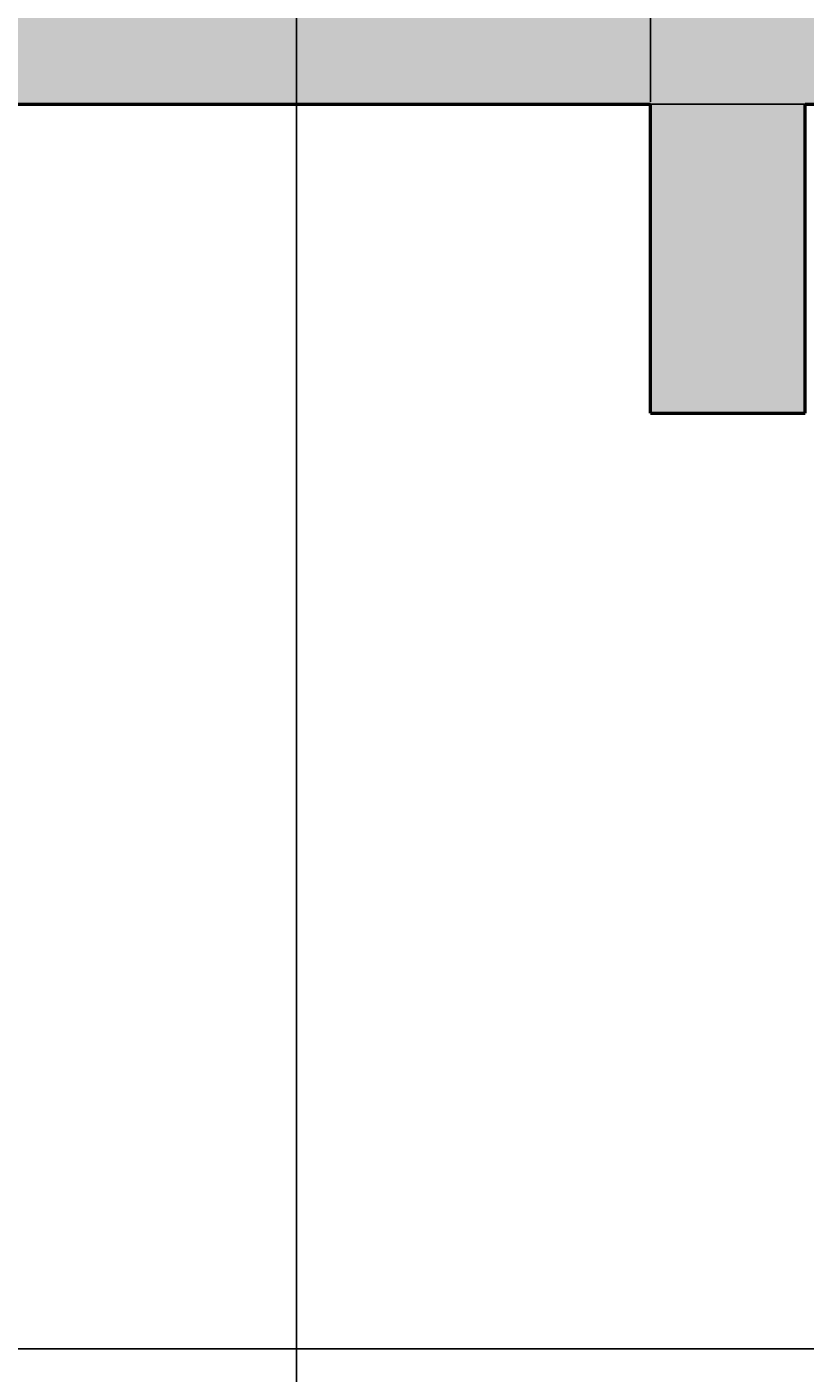
# Model space of a CAD drawing. Units: inches. Extents: x 2231 to 2461, y 2045 to 2455.
# Tile 10 of 95: x 2279 to 2299, y 2150 to 2185. Entities that reach past the tile are written whole.
import ezdxf

# ---------------------------------------------------------------- set-up
doc = ezdxf.new("R2010")
doc.units = ezdxf.units.IN
doc.layers.add('A-ANNO-DIMS', color=2, linetype='Continuous', lineweight=18)
doc.layers.add('A-WALL', color=7, linetype='Continuous', lineweight=50)
doc.layers.add('A-WALL-PATT', color=18, linetype='Continuous', lineweight=13, true_color=0x000000)
doc.styles.get("Standard").update_dxf_attribs({"font": 'arial.ttf'})
doc.dimstyles.get("Standard").update_dxf_attribs({"dimtxt": 0.18, "dimasz": 0.18, "dimexe": 0.18, "dimexo": 0.0625, "dimgap": 0.09, "dimtad": 0, "dimtih": 1, "dimtoh": 1, "dimdec": 4, "dimzin": 0, "dimdsep": 46, "dimtxsty": 'Standard', "dimcen": 0.09, "dimadec": 0, "dimazin": 0, "dimtfac": 1, "dimtdec": 4, "dimtofl": 0, "dimtmove": 0, "dimatfit": 3, "dimfxl": 1, "dimtolj": 1, "dimtzin": 0, "dimarcsym": 0})

# ---------------------------------------------------------------- blocks, each defined once
blk = doc.blocks.new('*D47')
at = {"layer": 'A-ANNO-DIMS', "color": 0, "lineweight": -2, "transparency": 16777216}
for p, q in [((2258.794, 2182.895), (2258.794, 2454.645)), ((2258.974, 2454.465), (2276.575, 2454.465)), ((2294.614, 2454.465), (2277.012, 2454.465)), ((2294.794, 2182.895), (2294.794, 2454.645))]:
    blk.add_line(p, q, dxfattribs=at)
at = {"layer": 'A-ANNO-DIMS', "color": 0, "transparency": 16777216}
for points in [[(2258.974, 2454.495), (2258.974, 2454.435), (2258.794, 2454.465)], [(2294.614, 2454.495), (2294.614, 2454.435), (2294.794, 2454.465)]]:
    blk.add_solid(points, dxfattribs=at)
at = {"layer": 'Defpoints', "color": 0, "transparency": 16777216}
for p in [(2294.794, 2454.465), (2258.794, 2182.833), (2294.794, 2182.833)]:
    blk.add_point(p, dxfattribs=at)
at = {"layer": 'A-ANNO-DIMS', "color": 0, "transparency": 16777216, "insert": (2276.794, 2454.465), "char_height": 0.18, "attachment_point": 5}
blk.add_mtext('\\A1;36', dxfattribs=at)
blk = doc.blocks.new('*D51')
at = {"layer": 'A-ANNO-DIMS', "color": 0, "lineweight": -2, "transparency": 16777216}
for p, q in [((2258.794, 2306.77), (2258.794, 2044.803)), ((2330.794, 2306.77), (2330.794, 2044.803)), ((2258.974, 2044.983), (2294.576, 2044.983)), ((2330.614, 2044.983), (2295.011, 2044.983))]:
    blk.add_line(p, q, dxfattribs=at)
at = {"layer": 'A-ANNO-DIMS', "color": 0, "transparency": 16777216}
for points in [[(2258.974, 2045.013), (2258.974, 2044.953), (2258.794, 2044.983)], [(2330.614, 2045.013), (2330.614, 2044.953), (2330.794, 2044.983)]]:
    blk.add_solid(points, dxfattribs=at)
at = {"layer": 'Defpoints', "color": 0, "transparency": 16777216}
for p in [(2258.794, 2306.833), (2330.794, 2306.833), (2330.794, 2044.983)]:
    blk.add_point(p, dxfattribs=at)
at = {"layer": 'A-ANNO-DIMS', "color": 0, "transparency": 16777216, "insert": (2294.794, 2044.983), "char_height": 0.18, "attachment_point": 5}
blk.add_mtext('\\A1;72', dxfattribs=at)
blk = doc.blocks.new('*D60')
at = {"layer": 'A-ANNO-DIMS', "color": 0, "lineweight": -2, "transparency": 16777216}
for p, q in [((2432.731, 2182.833), (2230.981, 2182.833)), ((2231.161, 2182.653), (2231.161, 2166.906)), ((2231.161, 2150.795), (2231.161, 2166.542)), ((2432.731, 2150.615), (2230.981, 2150.615))]:
    blk.add_line(p, q, dxfattribs=at)
at = {"layer": 'A-ANNO-DIMS', "color": 0, "transparency": 16777216}
for points in [[(2231.131, 2182.653), (2231.191, 2182.653), (2231.161, 2182.833)], [(2231.131, 2150.795), (2231.191, 2150.795), (2231.161, 2150.615)]]:
    blk.add_solid(points, dxfattribs=at)
at = {"layer": 'Defpoints', "color": 0, "transparency": 16777216}
for p in [(2231.161, 2182.833), (2432.794, 2182.833), (2432.794, 2150.615)]:
    blk.add_point(p, dxfattribs=at)
at = {"layer": 'A-ANNO-DIMS', "color": 0, "transparency": 16777216, "insert": (2231.161, 2166.724), "char_height": 0.18, "attachment_point": 5}
blk.add_mtext('\\A1;32.22', dxfattribs=at)
blk = doc.blocks.new('*D65')
at = {"layer": 'A-ANNO-DIMS', "color": 0, "lineweight": -2, "transparency": 16777216}
for p, q in [((2285.635, 2189.285), (2285.635, 2044.803)), ((2340.667, 2189.285), (2340.667, 2044.803)), ((2285.815, 2044.983), (2312.758, 2044.983)), ((2340.487, 2044.983), (2313.545, 2044.983))]:
    blk.add_line(p, q, dxfattribs=at)
at = {"layer": 'A-ANNO-DIMS', "color": 0, "transparency": 16777216}
for points in [[(2285.815, 2045.013), (2285.815, 2044.953), (2285.635, 2044.983)], [(2340.487, 2045.013), (2340.487, 2044.953), (2340.667, 2044.983)]]:
    blk.add_solid(points, dxfattribs=at)
at = {"layer": 'Defpoints', "color": 0, "transparency": 16777216}
for p in [(2285.635, 2189.348), (2340.667, 2189.348), (2340.667, 2044.983)]:
    blk.add_point(p, dxfattribs=at)
at = {"layer": 'A-ANNO-DIMS', "color": 0, "transparency": 16777216, "insert": (2313.151, 2044.983), "char_height": 0.18, "attachment_point": 5}
blk.add_mtext('\\A1;55.03', dxfattribs=at)

msp = doc.modelspace()

# ---------------------------------------------------------------- hatches: boundary and pattern name
at = {"layer": 'A-WALL-PATT'}
h = msp.add_hatch(color=256, dxfattribs=at)
h.dxf.hatch_style = 1
h.paths.add_polyline_path([(2441.7935, 2269.1535), (2432.7935, 2269.1535), (2432.7935, 2186.8328), (2396.7935, 2186.8328), (2396.7935, 2286.8328), (2394.7935, 2286.8328), (2394.7935, 2186.8328), (2334.7935, 2186.8328), (2334.7935, 2182.8328), (2432.7935, 2182.8328), (2432.7935, 2072.8328), (2416.6639, 2072.8328), (2416.6639, 2063.8328), (2441.7935, 2063.8328)])
h.paths.add_polyline_path([(2368.6639, 2072.8328), (2367.04, 2072.8328), (2330.7942, 2072.8328), (2330.7397, 2063.8328), (2368.6639, 2063.8328)])
h.paths.add_polyline_path([(2300.7392, 2068.3328), (2300.7392, 2072.8328), (2298.7935, 2072.8328), (2294.7935, 2072.8328), (2258.7935, 2072.8328), (2258.7935, 2120.8328), (2294.7935, 2120.8328), (2298.7935, 2120.8328), (2298.7935, 2128.8328), (2294.7935, 2128.8328), (2294.7935, 2124.8328), (2258.7935, 2124.8328), (2258.7935, 2182.8328), (2294.7935, 2182.8328), (2294.7935, 2174.8328), (2298.7935, 2174.8328), (2298.7935, 2182.8328), (2304.7935, 2182.8328), (2304.7935, 2186.8328), (2258.7935, 2186.8328), (2258.7935, 2221.999), (2249.7935, 2221.999), (2249.7935, 2063.8328), (2300.7392, 2063.8328)])
h.paths.add_polyline_path([(2391.9338, 2435.8328), (2333.82, 2435.8328), (2333.82, 2426.8328), (2368.7935, 2426.8328), (2368.7935, 2374.9508), (2368.7935, 2370.8328), (2372.3935, 2370.8328), (2372.7935, 2370.8328), (2372.7935, 2426.8328), (2391.9338, 2426.8328)])
h.paths.add_polyline_path([(2441.7935, 2435.8328), (2415.9338, 2435.8328), (2415.9338, 2426.8328), (2432.7935, 2426.8328), (2432.7935, 2334.8328), (2372.7935, 2334.8328), (2372.7935, 2346.8328), (2368.7935, 2346.8328), (2368.7935, 2306.8328), (2360.7935, 2306.8328), (2360.7935, 2302.8328), (2368.7935, 2302.8328), (2372.7935, 2302.8328), (2372.7935, 2330.8328), (2432.7935, 2330.8328), (2432.7935, 2317.1535), (2441.7935, 2317.1535)])
h.paths.add_polyline_path([(2285.82, 2435.8328), (2249.7935, 2435.8328), (2249.7935, 2269.999), (2258.7935, 2269.999), (2258.7935, 2302.8328), (2318.8168, 2302.8328), (2330.7935, 2302.8328), (2330.7935, 2306.8328), (2258.7935, 2306.8328), (2258.7935, 2426.8328), (2285.82, 2426.8328)])

# ---------------------------------------------------------------- linework, layer by layer
at = {"layer": 'A-WALL'}
for p, q in [((2258.7935, 2182.8328), (2294.7935, 2182.8328)), ((2294.7935, 2174.8328), (2294.7935, 2182.8328)), ((2298.7935, 2182.8328), (2304.7935, 2182.8328)), ((2298.7935, 2174.8328), (2298.7935, 2182.8328)), ((2294.7935, 2174.8328), (2298.7935, 2174.8328))]:
    msp.add_line(p, q, dxfattribs=at)

# ---------------------------------------------------------------- dimensions: what is measured, and where the dimension line sits
at = {"layer": 'A-ANNO-DIMS'}
for base, p1, p2, override, picture, middle in [((2294.7935, 2454.4653), (2258.7935, 2182.8328), (2294.7935, 2182.8328), {"dimdec": 0, "dimlfac": 1, "dimrnd": 0, "dimzin": 0, "dimdsep": 46, "dimlunit": 2}, '*D47', (2276.7935, 2454.4653)), ((2330.7935, 2044.9825), (2258.7935, 2306.8328), (2330.7935, 2306.8328), {"dimdec": 0, "dimlfac": 1, "dimrnd": 0, "dimzin": 0, "dimdsep": 46, "dimlunit": 2}, '*D51', (2294.7935, 2044.9825)), ((2340.6673, 2044.9825), (2285.6353, 2189.3477), (2340.6673, 2189.3477), {"dimdec": 2, "dimlfac": 1, "dimrnd": 0, "dimzin": 0, "dimdsep": 46, "dimlunit": 2}, '*D65', (2313.1513, 2044.9825))]:
    dim = msp.add_linear_dim(base=base, p1=p1, p2=p2, dimstyle='Standard', override=override, dxfattribs=at)
    dim.commit()
    dim.dimension.update_dxf_attribs({"geometry": picture, "text_midpoint": middle})
dim = msp.add_linear_dim(base=(2231.161, 2182.8328), p1=(2432.7935, 2150.6145), p2=(2432.7935, 2182.8328), angle=90, dimstyle='Standard', override={"dimdec": 2, "dimlfac": 1, "dimrnd": 0, "dimzin": 0, "dimdsep": 46, "dimlunit": 2}, dxfattribs=at)
dim.commit()
dim.dimension.update_dxf_attribs({"geometry": '*D60', "text_midpoint": (2231.161, 2166.7237)})

doc.saveas('drawing.dxf')
